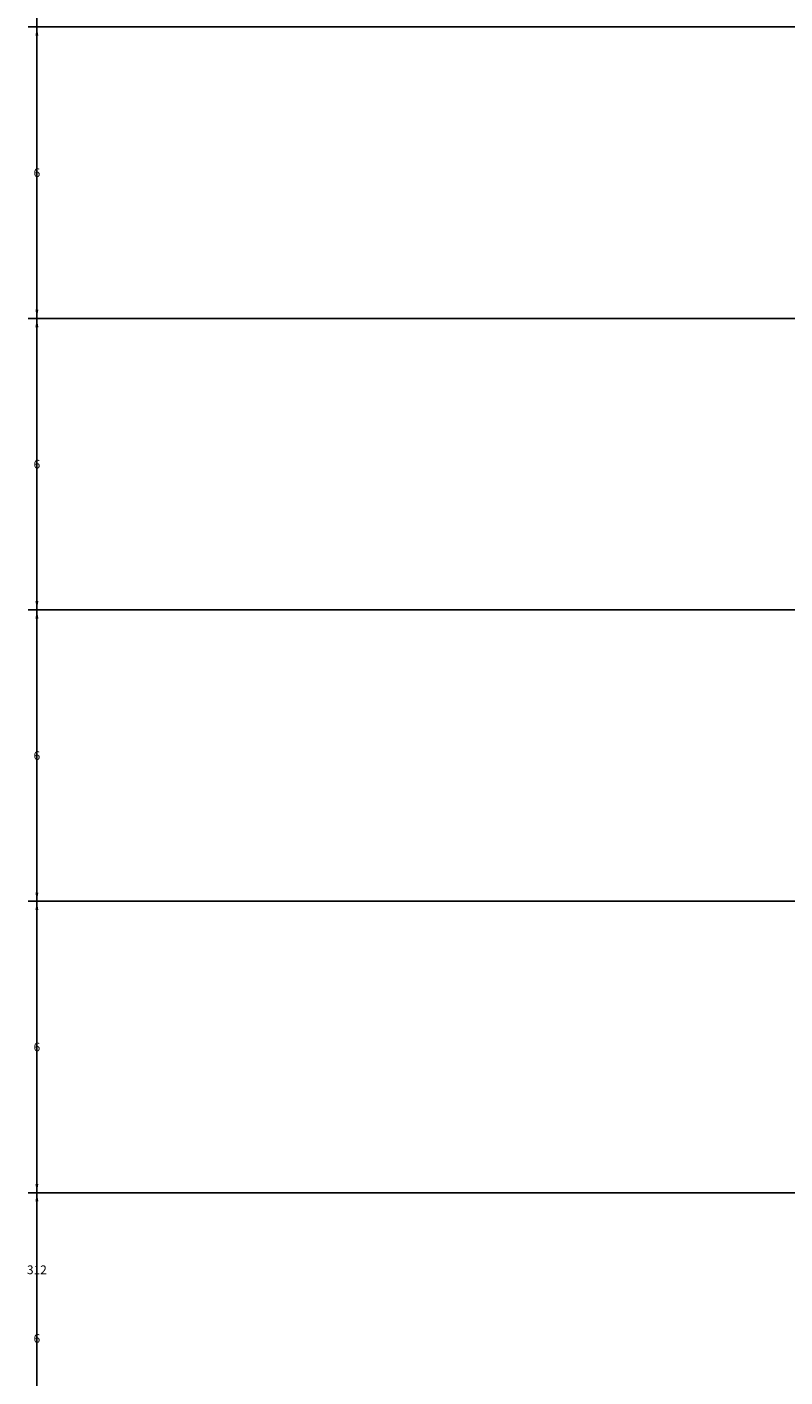
# Model space of a CAD drawing. Units: feet. Extents: x 2695 to 2912, y 795 to 1139.
# Tile 37 of 83: x 2695 to 2710, y 965 to 993. Entities that reach past the tile are written whole.
import ezdxf

# ---------------------------------------------------------------- set-up
doc = ezdxf.new("R2010")
doc.units = ezdxf.units.FT
doc.layers.add('A-ANNO-DIMS', color=2, linetype='Continuous', lineweight=18)
doc.styles.get("Standard").update_dxf_attribs({"font": 'arial.ttf'})
doc.dimstyles.get("Standard").update_dxf_attribs({"dimtxt": 0.18, "dimasz": 0.18, "dimexe": 0.18, "dimexo": 0.0625, "dimgap": 0.09, "dimtad": 0, "dimtih": 1, "dimtoh": 1, "dimdec": 1, "dimzin": 0, "dimdsep": 46, "dimlunit": 3, "dimtxsty": 'Standard', "dimcen": 0.09, "dimadec": 0, "dimazin": 0, "dimtfac": 1, "dimtdec": 1, "dimtofl": 0, "dimtmove": 0, "dimatfit": 3, "dimfxl": 1, "dimtolj": 1, "dimtzin": 0, "dimarcsym": 0})

# ---------------------------------------------------------------- blocks, each defined once
blk = doc.blocks.new('*D12')
at = {"layer": 'A-ANNO-DIMS', "color": 0, "lineweight": -2, "transparency": 16777216}
for p, q in [((2710.574, 1122.931), (2694.681, 1122.931)), ((2694.861, 1122.751), (2694.861, 967.113)), ((2694.861, 811.111), (2694.861, 966.749)), ((2710.574, 810.931), (2694.681, 810.931))]:
    blk.add_line(p, q, dxfattribs=at)
at = {"layer": 'A-ANNO-DIMS', "color": 0, "transparency": 16777216}
for points in [[(2694.831, 1122.751), (2694.891, 1122.751), (2694.861, 1122.931)], [(2694.831, 811.111), (2694.891, 811.111), (2694.861, 810.931)]]:
    blk.add_solid(points, dxfattribs=at)
at = {"layer": 'Defpoints', "color": 0, "transparency": 16777216}
for p in [(2694.861, 1122.931), (2710.636, 1122.931), (2710.636, 810.931)]:
    blk.add_point(p, dxfattribs=at)
at = {"layer": 'A-ANNO-DIMS', "color": 0, "transparency": 16777216, "insert": (2694.861, 966.931), "char_height": 0.18, "attachment_point": 5}
blk.add_mtext('\\A1;312', dxfattribs=at)
blk = doc.blocks.new('*D32')
at = {"layer": 'A-ANNO-DIMS', "color": 0, "lineweight": -2, "transparency": 16777216}
for p, q in [((2730.646, 968.518), (2694.681, 968.518)), ((2694.861, 968.338), (2694.861, 965.7)), ((2694.861, 962.698), (2694.861, 965.336)), ((2730.646, 962.518), (2694.681, 962.518))]:
    blk.add_line(p, q, dxfattribs=at)
at = {"layer": 'A-ANNO-DIMS', "color": 0, "transparency": 16777216}
for points in [[(2694.831, 968.338), (2694.891, 968.338), (2694.861, 968.518)], [(2694.831, 962.698), (2694.891, 962.698), (2694.861, 962.518)]]:
    blk.add_solid(points, dxfattribs=at)
at = {"layer": 'Defpoints', "color": 0, "transparency": 16777216}
for p in [(2694.861, 968.518), (2730.708, 968.518), (2730.708, 962.518)]:
    blk.add_point(p, dxfattribs=at)
at = {"layer": 'A-ANNO-DIMS', "color": 0, "transparency": 16777216, "insert": (2694.861, 965.518), "char_height": 0.18, "attachment_point": 5}
blk.add_mtext('\\A1;6', dxfattribs=at)
blk = doc.blocks.new('*D33')
at = {"layer": 'A-ANNO-DIMS', "color": 0, "lineweight": -2, "transparency": 16777216}
for p, q in [((2730.646, 974.518), (2694.681, 974.518)), ((2694.861, 974.338), (2694.861, 971.7)), ((2694.861, 968.698), (2694.861, 971.336)), ((2730.646, 968.518), (2694.681, 968.518))]:
    blk.add_line(p, q, dxfattribs=at)
at = {"layer": 'A-ANNO-DIMS', "color": 0, "transparency": 16777216}
for points in [[(2694.831, 974.338), (2694.891, 974.338), (2694.861, 974.518)], [(2694.831, 968.698), (2694.891, 968.698), (2694.861, 968.518)]]:
    blk.add_solid(points, dxfattribs=at)
at = {"layer": 'Defpoints', "color": 0, "transparency": 16777216}
for p in [(2694.861, 974.518), (2730.708, 974.518), (2730.708, 968.518)]:
    blk.add_point(p, dxfattribs=at)
at = {"layer": 'A-ANNO-DIMS', "color": 0, "transparency": 16777216, "insert": (2694.861, 971.518), "char_height": 0.18, "attachment_point": 5}
blk.add_mtext('\\A1;6', dxfattribs=at)
blk = doc.blocks.new('*D34')
at = {"layer": 'A-ANNO-DIMS', "color": 0, "lineweight": -2, "transparency": 16777216}
for p, q in [((2730.646, 980.518), (2694.681, 980.518)), ((2694.861, 980.338), (2694.861, 977.7)), ((2694.861, 974.698), (2694.861, 977.336)), ((2730.646, 974.518), (2694.681, 974.518))]:
    blk.add_line(p, q, dxfattribs=at)
at = {"layer": 'A-ANNO-DIMS', "color": 0, "transparency": 16777216}
for points in [[(2694.831, 980.338), (2694.891, 980.338), (2694.861, 980.518)], [(2694.831, 974.698), (2694.891, 974.698), (2694.861, 974.518)]]:
    blk.add_solid(points, dxfattribs=at)
at = {"layer": 'Defpoints', "color": 0, "transparency": 16777216}
for p in [(2694.861, 980.518), (2730.708, 980.518), (2730.708, 974.518)]:
    blk.add_point(p, dxfattribs=at)
at = {"layer": 'A-ANNO-DIMS', "color": 0, "transparency": 16777216, "insert": (2694.861, 977.518), "char_height": 0.18, "attachment_point": 5}
blk.add_mtext('\\A1;6', dxfattribs=at)
blk = doc.blocks.new('*D35')
at = {"layer": 'A-ANNO-DIMS', "color": 0, "lineweight": -2, "transparency": 16777216}
for p, q in [((2730.646, 986.518), (2694.681, 986.518)), ((2694.861, 986.338), (2694.861, 983.7)), ((2694.861, 980.698), (2694.861, 983.336)), ((2730.646, 980.518), (2694.681, 980.518))]:
    blk.add_line(p, q, dxfattribs=at)
at = {"layer": 'A-ANNO-DIMS', "color": 0, "transparency": 16777216}
for points in [[(2694.831, 986.338), (2694.891, 986.338), (2694.861, 986.518)], [(2694.831, 980.698), (2694.891, 980.698), (2694.861, 980.518)]]:
    blk.add_solid(points, dxfattribs=at)
at = {"layer": 'Defpoints', "color": 0, "transparency": 16777216}
for p in [(2694.861, 986.518), (2730.708, 986.518), (2730.708, 980.518)]:
    blk.add_point(p, dxfattribs=at)
at = {"layer": 'A-ANNO-DIMS', "color": 0, "transparency": 16777216, "insert": (2694.861, 983.518), "char_height": 0.18, "attachment_point": 5}
blk.add_mtext('\\A1;6', dxfattribs=at)
blk = doc.blocks.new('*D36')
at = {"layer": 'A-ANNO-DIMS', "color": 0, "lineweight": -2, "transparency": 16777216}
for p, q in [((2730.646, 992.518), (2694.681, 992.518)), ((2694.861, 992.338), (2694.861, 989.7)), ((2694.861, 986.698), (2694.861, 989.336)), ((2730.646, 986.518), (2694.681, 986.518))]:
    blk.add_line(p, q, dxfattribs=at)
at = {"layer": 'A-ANNO-DIMS', "color": 0, "transparency": 16777216}
for points in [[(2694.831, 992.338), (2694.891, 992.338), (2694.861, 992.518)], [(2694.831, 986.698), (2694.891, 986.698), (2694.861, 986.518)]]:
    blk.add_solid(points, dxfattribs=at)
at = {"layer": 'Defpoints', "color": 0, "transparency": 16777216}
for p in [(2694.861, 992.518), (2730.708, 992.518), (2730.708, 986.518)]:
    blk.add_point(p, dxfattribs=at)
at = {"layer": 'A-ANNO-DIMS', "color": 0, "transparency": 16777216, "insert": (2694.861, 989.518), "char_height": 0.18, "attachment_point": 5}
blk.add_mtext('\\A1;6', dxfattribs=at)

msp = doc.modelspace()

# ---------------------------------------------------------------- dimensions: what is measured, and where the dimension line sits
at = {"layer": 'A-ANNO-DIMS'}
for base, p1, p2, picture, middle in [((2694.8611, 1122.9306), (2710.6361, 810.9306), (2710.6361, 1122.9306), '*D12', (2694.8611, 966.9306)), ((2694.8611, 992.5179), (2730.7081, 986.5179), (2730.7081, 992.5179), '*D36', (2694.8611, 989.5179)), ((2694.8611, 986.5179), (2730.7081, 980.5179), (2730.7081, 986.5179), '*D35', (2694.8611, 983.5179)), ((2694.8611, 980.5179), (2730.7081, 974.5179), (2730.7081, 980.5179), '*D34', (2694.8611, 977.5179)), ((2694.8611, 974.5179), (2730.7081, 968.5179), (2730.7081, 974.5179), '*D33', (2694.8611, 971.5179)), ((2694.8611, 968.5179), (2730.7081, 962.5179), (2730.7081, 968.5179), '*D32', (2694.8611, 965.5179))]:
    dim = msp.add_linear_dim(base=base, p1=p1, p2=p2, angle=90, dimstyle='Standard', override={"dimdec": 0, "dimlfac": 1, "dimrnd": 0, "dimzin": 0, "dimdsep": 46, "dimlunit": 2}, dxfattribs=at)
    dim.commit()
    dim.dimension.update_dxf_attribs({"geometry": picture, "text_midpoint": middle})

doc.saveas('drawing.dxf')
